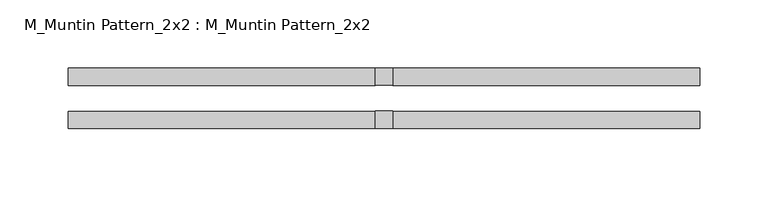
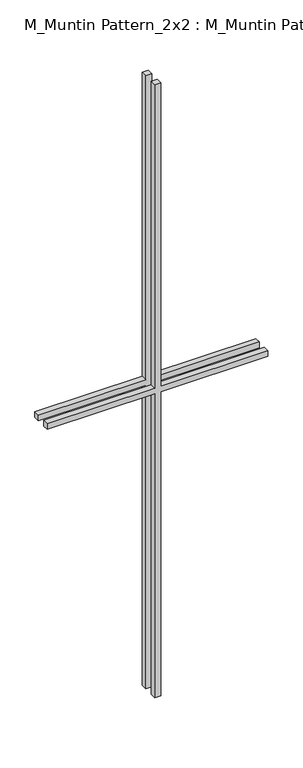
"""IFC4 building model written with IfcOpenShell, lengths in millimetres: proxy geometry, M_Muntin Pattern_2x2 : M_Muntin Pattern_2x2."""

from ifc_helpers import new_model, si_unit, frame, origin, place, context, project, spatial, polyline, outline, extrude, source, transform, mapped, element, save


def m_muntin_pattern_2x2_m_muntin_pattern_2x2_dce6eb8c(model_context):
    return source(origin(), model_context, "Body", "SweptSolid", [
        extrude(outline(polyline([(686.5, -6.35), (686.5, -231.7375), (673.8, -231.7375), (673.8, -6.35), (0.0, -6.35), (0.0, 6.35), (673.8, 6.35), (673.8, 231.7375), (686.5, 231.7375), (686.5, 6.35), (1360.3, 6.35), (1360.3, -6.35), (686.5, -6.35)])), frame((0.0, -22.225, 0.0), z_axis=(0.0, 1.0, 0.0), x_axis=(0.0, 0.0, 1.0)), (0.0, 0.0, 1.0), 12.7),
        extrude(outline(polyline([(686.5, -6.35), (686.5, -231.7375), (673.8, -231.7375), (673.8, -6.35), (0.0, -6.35), (0.0, 6.35), (673.8, 6.35), (673.8, 231.7375), (686.5, 231.7375), (686.5, 6.35), (1360.3, 6.35), (1360.3, -6.35), (686.5, -6.35)])), frame((0.0, 9.525, 0.0), z_axis=(0.0, 1.0, 0.0), x_axis=(0.0, 0.0, 1.0)), (0.0, 0.0, 1.0), 12.7),
    ])


if __name__ == "__main__":
    model = new_model("IFC4")
    model_context = context("Model", 3, world=origin())
    ifc_project = project(units=[si_unit("LENGTHUNIT", "METRE", prefix="MILLI")], contexts=[model_context])
    site = spatial("IfcSite", under=ifc_project)
    building = spatial("IfcBuilding", under=site)
    placement = place(None, origin())
    m_muntin_pattern_2x2_m_muntin_pattern_2x2_shape = m_muntin_pattern_2x2_m_muntin_pattern_2x2_dce6eb8c(model_context)
    element("IfcBuildingElementProxy", 1, Name="M_Muntin Pattern_2x2 : M_Muntin Pattern_2x2", ObjectType="M_Muntin Pattern_2x2 : M_Muntin Pattern_2x2", at=placement, inside=building, context=model_context, shape_type="MappedRepresentation", body=[
        mapped(m_muntin_pattern_2x2_m_muntin_pattern_2x2_shape, transform((0.0, 0.0, 0.0), x_axis=(1.0, 0.0, 0.0), y_axis=(0.0, 1.0, 0.0), z_axis=(0.0, 0.0, 1.0))),
    ])
    save(model, "model.ifc")

# Revit data of these elements
# Type "M_Muntin Pattern_2x2 : M_Muntin Pattern_2x2"
#   Width [instance default] = 3.937008 ft
#   Thickness = 0.041667 ft
#   Height [instance default] = 3.937008 ft
#   Distance = 0.0625 ft
#   Interior Material [instance default] = none
#   Exterior Material [instance default] = none
#   Default Elevation = 0
# Element 1 (IfcBuildingElementProxy, "M_Muntin Pattern_2x2 : M_Muntin Pattern_2x2")
#   Width = 1.520587 ft
#   Height = 4.462927 ft
#   Interior Material = Wood - Stained
#   Exterior Material = Clad - White
#   Materials on its faces: "Clad - White", "Wood - Stained"
# Materials
#   "Clad - White": class "Wood", colour RGB 242 242 238, transparency 0, Cost = 0
#   "Wood - Stained": class "Wood", colour RGB 224 178 126, transparency 0, Cost = 0
